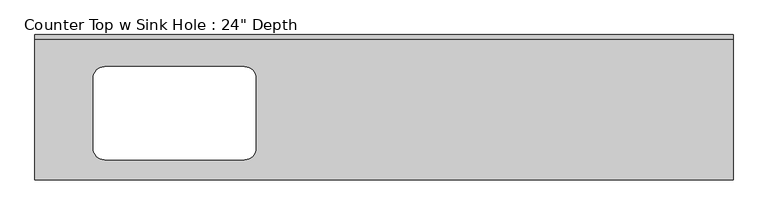
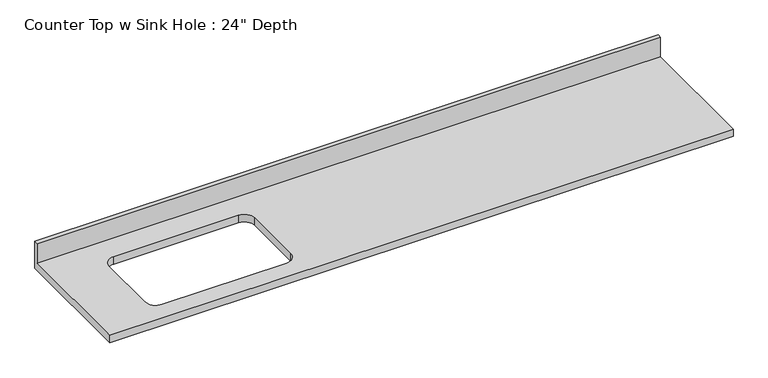
"""IFC4 building model written with IfcOpenShell, lengths in millimetres: furniture geometry."""

from ifc_helpers import new_model, si_unit, frame, origin, place, context, project, spatial, polyline, circle_curve, source, transform, mapped, element, save
from ifc_brep_helpers import plane_surface, revolved_surface, advanced_brep


def furniture_771c7099(model_context):
    return source(origin(), model_context, "Body", "AdvancedBrep", [
        advanced_brep(
        [(-1200.4622951, -635.0, 914.4), (1847.5377049, -635.0, 914.4), (1847.5377049, -19.05, 914.4), (-1200.4622951, -19.05, 914.4), (-895.6622951, -139.7, 914.4), (-286.0622951, -139.7, 914.4), (-235.2622951, -190.5, 914.4), (-235.2622951, -495.3, 914.4), (-286.0622951, -546.1, 914.4), (-895.6622951, -546.1, 914.4), (-946.4622951, -495.3, 914.4), (-946.4622951, -190.5, 914.4), (1847.5377049, 0.0, 876.3), (1847.5377049, -635.0, 876.3), (-1200.4622951, -635.0, 876.3), (-1200.4622951, 0.0, 876.3), (-286.0622951, -139.7, 876.3), (-895.6622951, -139.7, 876.3), (-946.4622951, -190.5, 876.3), (-946.4622951, -495.3, 876.3), (-895.6622951, -546.1, 876.3), (-286.0622951, -546.1, 876.3), (-235.2622951, -495.3, 876.3), (-235.2622951, -190.5, 876.3), (-1200.4622951, 0.0, 1016.0), (1847.5377049, 0.0, 1016.0), (-1200.4622951, -19.05, 1016.0), (1847.5377049, -19.05, 1016.0)],
        [
            (0, 1),
            (1, 2),
            (2, 3),
            (3, 0),
            (4, 5),
            (5, 6, circle_curve(frame((-286.0622951, -190.5, 914.4), z_axis=(0.0, 0.0, -1.0), x_axis=(1.0, 0.0, 0.0)), 50.8)),
            (6, 7),
            (7, 8, circle_curve(frame((-286.0622951, -495.3, 914.4), z_axis=(0.0, 0.0, -1.0), x_axis=(1.0, 0.0, 0.0)), 50.8)),
            (8, 9),
            (9, 10, circle_curve(frame((-895.6622951, -495.3, 914.4), z_axis=(0.0, 0.0, -1.0), x_axis=(1.0, 0.0, 0.0)), 50.8)),
            (10, 11),
            (11, 4, circle_curve(frame((-895.6622951, -190.5, 914.4), z_axis=(0.0, 0.0, -1.0), x_axis=(1.0, 0.0, 0.0)), 50.8)),
            (12, 13),
            (13, 14),
            (14, 15),
            (15, 12),
            (16, 17),
            (17, 18, circle_curve(frame((-895.6622951, -190.5, 876.3), z_axis=(0.0, 0.0, 1.0), x_axis=(1.0, 0.0, 0.0)), 50.8)),
            (18, 19),
            (19, 20, circle_curve(frame((-895.6622951, -495.3, 876.3), z_axis=(0.0, 0.0, 1.0), x_axis=(1.0, 0.0, 0.0)), 50.8)),
            (20, 21),
            (21, 22, circle_curve(frame((-286.0622951, -495.3, 876.3), z_axis=(0.0, 0.0, 1.0), x_axis=(1.0, 0.0, 0.0)), 50.8)),
            (22, 23),
            (23, 16, circle_curve(frame((-286.0622951, -190.5, 876.3), z_axis=(0.0, 0.0, 1.0), x_axis=(1.0, 0.0, 0.0)), 50.8)),
            (15, 24),
            (24, 25),
            (25, 12),
            (14, 0),
            (3, 26),
            (26, 24),
            (13, 1),
            (25, 27),
            (27, 2),
            (26, 27),
            (4, 17),
            (16, 5),
            (11, 18),
            (10, 19),
            (9, 20),
            (8, 21),
            (7, 22),
            (6, 23),
        ],
        [
            plane_surface(frame((-1200.4622951, 0.0, 914.4), z_axis=(0.0, 0.0, 1.0), x_axis=(-1.0, 0.0, 0.0))),
            plane_surface(frame((-1200.4622951, 0.0, 876.3), z_axis=(0.0, 0.0, -1.0), x_axis=(1.0, 0.0, 0.0))),
            plane_surface(frame((1847.5377049, 0.0, 914.4), z_axis=(0.0, 1.0, 0.0), x_axis=(0.0, 0.0, -1.0))),
            plane_surface(frame((-1200.4622951, 0.0, 914.4), z_axis=(-1.0, 0.0, 0.0), x_axis=(0.0, 0.0, -1.0))),
            plane_surface(frame((-1200.4622951, -635.0, 914.4), z_axis=(0.0, -1.0, 0.0), x_axis=(0.0, 0.0, -1.0))),
            plane_surface(frame((1847.5377049, -635.0, 914.4), z_axis=(1.0, 0.0, 0.0), x_axis=(0.0, 0.0, -1.0))),
            plane_surface(frame((-1200.4622951, 0.0, 1016.0), z_axis=(0.0, 0.0, 1.0), x_axis=(0.0, -1.0, 0.0))),
            plane_surface(frame((-1200.4622951, -19.05, 1016.0), z_axis=(0.0, -1.0, 0.0), x_axis=(0.0, 0.0, -1.0))),
            plane_surface(frame((-286.0622951, -139.7, 914.4), z_axis=(0.0, -1.0, 0.0), x_axis=(0.0, 0.0, -1.0))),
            revolved_surface(polyline([(-844.8622951000001, -190.5, 914.4), (-844.8622951000001, -190.5, 876.3)]), (-895.6622951, -190.5, 876.3), (0.0, 0.0, 1.0)),
            plane_surface(frame((-946.4622951, -190.5, 914.4), z_axis=(1.0, 0.0, 0.0), x_axis=(0.0, 0.0, -1.0))),
            revolved_surface(polyline([(-844.8622951000001, -495.3, 914.4), (-844.8622951000001, -495.3, 876.3)]), (-895.6622951, -495.3, 876.3), (0.0, 0.0, 1.0)),
            plane_surface(frame((-895.6622951, -546.1, 914.4), z_axis=(0.0, 1.0, 0.0), x_axis=(0.0, 0.0, -1.0))),
            revolved_surface(polyline([(-235.26229509999996, -495.3, 914.4), (-235.26229509999996, -495.3, 876.3)]), (-286.0622951, -495.3, 876.3), (0.0, 0.0, 1.0)),
            plane_surface(frame((-235.2622951, -495.3, 914.4), z_axis=(-1.0, 0.0, 0.0), x_axis=(0.0, 0.0, -1.0))),
            revolved_surface(polyline([(-235.26229509999996, -190.5, 914.4), (-235.26229509999996, -190.5, 876.3)]), (-286.0622951, -190.5, 876.3), (0.0, 0.0, 1.0)),
        ],
        [
            (0, [[1, 2, 3, 4], [5, 6, 7, 8, 9, 10, 11, 12]]),
            (1, [[13, 14, 15, 16], [17, 18, 19, 20, 21, 22, 23, 24]]),
            (2, [[-16, 25, 26, 27]]),
            (3, [[-15, 28, -4, 29, 30, -25]]),
            (4, [[-1, -28, -14, 31]]),
            (5, [[-13, -27, 32, 33, -2, -31]]),
            (6, [[-30, 34, -32, -26]]),
            (7, [[-34, -29, -3, -33]]),
            (8, [[35, -17, 36, -5]]),
            (9, [[-35, -12, 37, -18]]),
            (10, [[-37, -11, 38, -19]]),
            (11, [[-38, -10, 39, -20]]),
            (12, [[-39, -9, 40, -21]]),
            (13, [[-40, -8, 41, -22]]),
            (14, [[-41, -7, 42, -23]]),
            (15, [[-36, -24, -42, -6]]),
        ],
    ),
    ])


if __name__ == "__main__":
    model = new_model("IFC4")
    model_context = context("Model", 3, world=origin())
    ifc_project = project(units=[si_unit("LENGTHUNIT", "METRE", prefix="MILLI")], contexts=[model_context])
    site = spatial("IfcSite", under=ifc_project)
    building = spatial("IfcBuilding", under=site)
    placement = place(None, origin())
    furniture_shape = furniture_771c7099(model_context)
    element("IfcFurniture", 1, ObjectType="Counter Top w Sink Hole : 24\" Depth", at=placement, inside=building, context=model_context, shape_type="MappedRepresentation", body=[
        mapped(furniture_shape, transform((0.0, 0.0, 0.0), x_axis=(1.0, 0.0, 0.0), y_axis=(0.0, 1.0, 0.0), z_axis=(0.0, 0.0, 1.0))),
    ])
    save(model, "model.ifc")

# Revit data of these elements
# Type "Counter Top w Sink Hole : 24\" Depth"
#   Assembly Code = "C1030400"
#   Counter Thickness = 0' - 1 1/2"
#   Depth = 2' - 1"
#   Height = 3' - 0"
#   Length [instance default] = 8' - 0"
#   Sink Location [instance default] = 2' - 0"
#   Sink Location To Wall [instance default] = 0' - 6"
#   Sink Opening Depth [instance default] = 1' - 3"
#   Sink Opening Width [instance default] = 2' - 3"
#   Counter Top Material = none
#   Default Elevation = 0
# Element 1 (IfcFurniture, "Counter Top w Sink Hole : 24\" Depth")
#   Length = 10' - 0"
#   Materials on its faces: "Counter Top"
# Materials
#   "Counter Top": class "Wood", colour RGB 226 177 128, transparency 0
